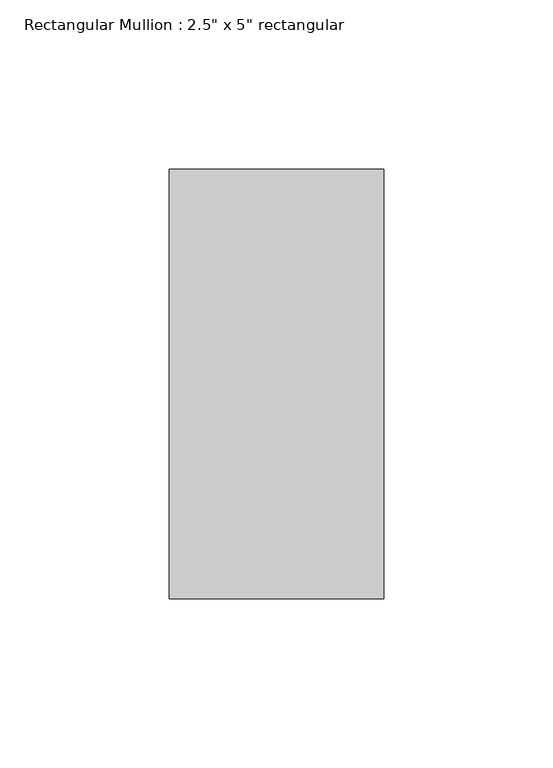
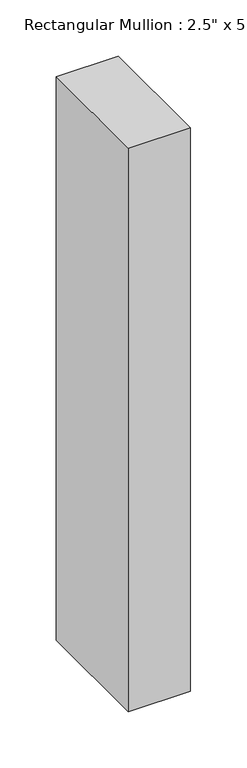
"""IFC4 building model written with IfcOpenShell, lengths in millimetres: member geometry."""

from ifc_helpers import new_model, si_unit, frame, origin, place, context, project, spatial, polyline, outline, extrude, source, transform, mapped, element, save


def member_6e77e263(model_context):
    return source(origin(), model_context, "Body", "SweptSolid", [
        extrude(outline(polyline([(31.75, 63.5), (31.75, -63.5), (-31.75, -63.5), (-31.75, 63.5), (31.75, 63.5)])), frame((0.0, 0.0, -609.6), z_axis=(0.0, 0.0, 1.0), x_axis=(1.0, 0.0, 0.0)), (0.0, 0.0, 1.0), 609.6),
    ])


if __name__ == "__main__":
    model = new_model("IFC4")
    model_context = context("Model", 3, world=origin())
    ifc_project = project(units=[si_unit("LENGTHUNIT", "METRE", prefix="MILLI")], contexts=[model_context])
    site = spatial("IfcSite", under=ifc_project)
    building = spatial("IfcBuilding", under=site)
    placement = place(None, origin())
    member_shape = member_6e77e263(model_context)
    element("IfcMember", 1, ObjectType="Rectangular Mullion : 2.5\" x 5\" rectangular", at=placement, inside=building, context=model_context, shape_type="MappedRepresentation", body=[
        mapped(member_shape, transform((0.0, 0.0, 0.0), x_axis=(1.0, 0.0, 0.0), y_axis=(0.0, 1.0, 0.0), z_axis=(0.0, 0.0, 1.0))),
    ])
    save(model, "model.ifc")

# Revit data of these elements
# Type "Rectangular Mullion : 2.5\" x 5\" rectangular"
#   built-in parameter 1007304 = 0.416667 (stored number, unit not read)
#   built-in parameter 1007301 = 0.104167 (stored number, unit not read)
#   built-in parameter 1007300 = 0.104167 (stored number, unit not read)
# Element 1 (IfcMember, "Rectangular Mullion : 2.5\" x 5\" rectangular")
#   Materials on its faces: "BLACK COLOUR"
# Materials
#   "BLACK COLOUR": class "Generic", colour RGB 120 120 120, transparency 0, Cost = 0
